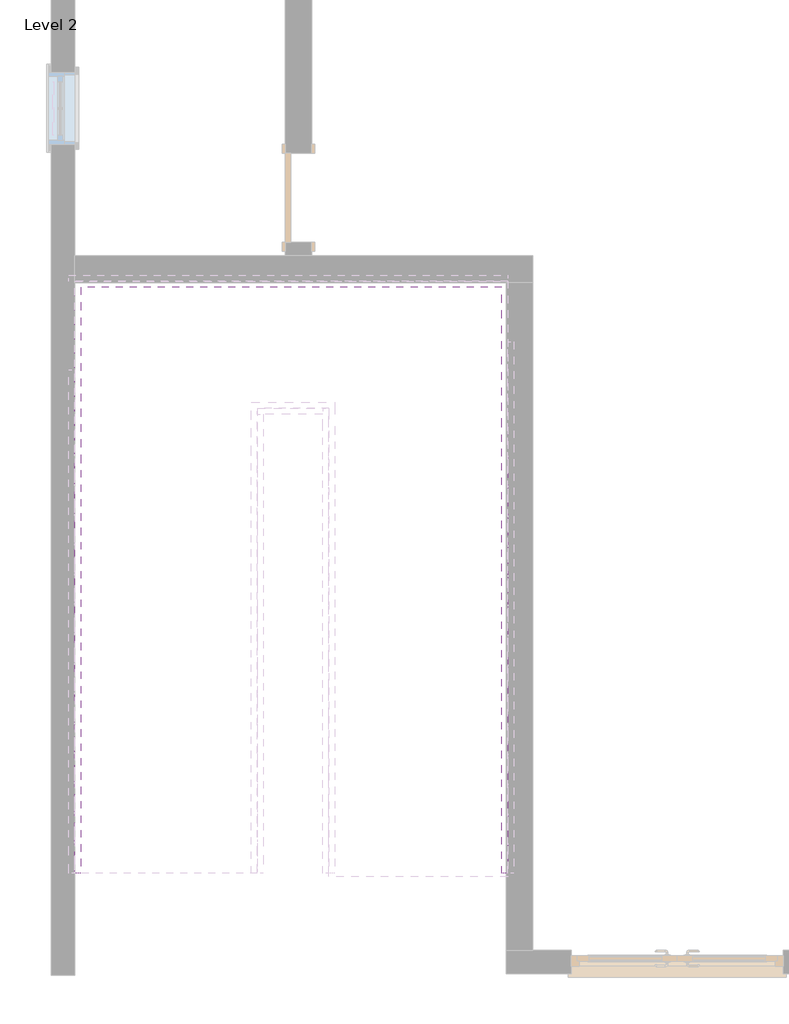
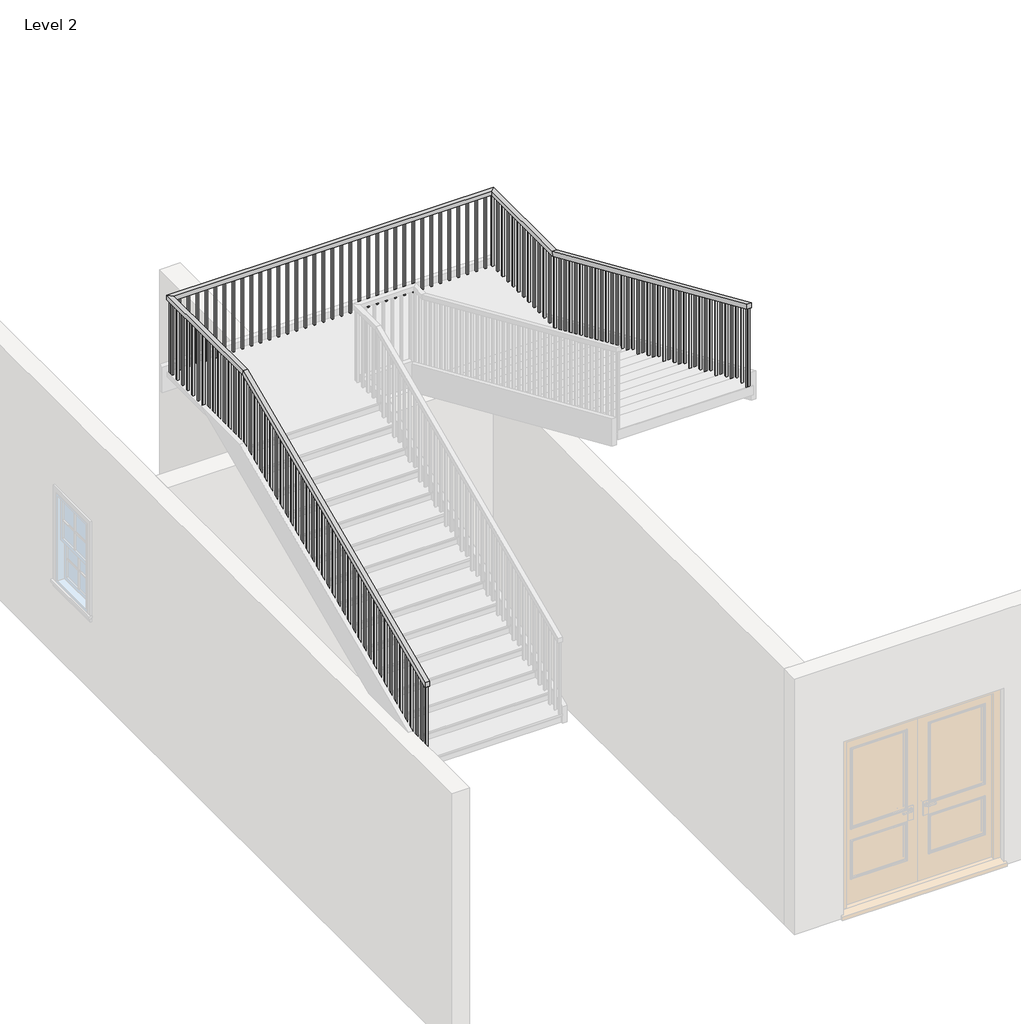
# One storey, part 3 of 4: 1 railing.
"""IFC4 building model written with IfcOpenShell, lengths in millimetres."""

from ifc_helpers import new_model, si_unit, frame, origin, place, context, project, spatial, polyline, outline, extrude, faceted_brep, element, save

model = new_model("IFC4")

# Units and contexts
model_context = context("Model", 3, world=origin())
ifc_project = project(units=[si_unit("LENGTHUNIT", "METRE", prefix="MILLI")], contexts=[model_context])

# Site, building, storey
site = spatial("IfcSite", under=ifc_project)
building = spatial("IfcBuilding", under=site)
storey = spatial("IfcBuildingStorey", under=building, Name="Level 2", Elevation=3048.0)

# Railing
placement = place(None, origin())
element("IfcRailing", 1, ObjectType="Handrail - Rectangular", at=placement, inside=storey, context=model_context, shape_type="SolidModel", body=[
    faceted_brep([(-7554.4415084, -6973.0610642, 6817.36), (-7554.4415084, -6973.0610642, 6761.8599828), (-7503.6415084, -6973.0610642, 6761.8599828), (-7503.6415084, -6973.0610642, 6817.36), (-7554.4415084, -3417.0610642, 8382.0), (-7554.4415084, -3406.3792071, 8331.2), (-7503.6415084, -3406.3792071, 8331.2), (-7503.6415084, -3417.0610642, 8382.0), (-7554.4415084, -1928.4217109, 8382.0), (-7554.4415084, -1928.4217109, 8331.2), (-7503.6415084, -1979.2217109, 8331.2), (-7503.6415084, -1979.2217109, 8382.0), (-3866.3290366, -1928.4217109, 8382.0), (-3866.3290366, -1928.4217109, 8331.2), (-3917.1290366, -1979.2217109, 8331.2), (-3917.1290366, -1979.2217109, 8382.0), (-3866.3290366, -3163.0610642, 8382.0), (-3866.3290366, -3173.7429214, 8331.2), (-3917.1290366, -3173.7429214, 8331.2), (-3917.1290366, -3163.0610642, 8382.0), (-3866.3290366, -6973.0610642, 10058.4), (-3917.1290366, -6973.0610642, 10058.4), (-3917.1290366, -6973.0610642, 10002.8999828), (-3866.3290366, -6973.0610642, 10002.8999828)], [[[0, 1, 2, 3]], [[1, 0, 4, 5]], [[2, 1, 5, 6]], [[3, 2, 6, 7]], [[0, 3, 7, 4]], [[5, 4, 8, 9]], [[6, 5, 9, 10]], [[7, 6, 10, 11]], [[4, 7, 11, 8]], [[9, 8, 12, 13]], [[10, 9, 13, 14]], [[11, 10, 14, 15]], [[8, 11, 15, 12]], [[13, 12, 16, 17]], [[14, 13, 17, 18]], [[15, 14, 18, 19]], [[12, 15, 19, 16]], [[20, 21, 22, 23]], [[17, 16, 20, 23]], [[18, 17, 23, 22]], [[19, 18, 22, 21]], [[16, 19, 21, 20]]]),
    extrude(outline(polyline([(-6922.6967109, 9980.7396674), (-6922.6967109, 9032.24), (-6941.7467109, 9032.24), (-6941.7467109, 9989.1216674), (-6922.6967109, 9980.7396674)])), frame((-3901.2540366, 0.0, 0.0), z_axis=(1.0, 0.0, 0.0), x_axis=(0.0, 1.0, 0.0)), (0.0, 0.0, 1.0), 19.05),
    extrude(outline(polyline([(-6821.0967109, 9936.0356674), (-6821.0967109, 9032.24), (-6840.1467109, 9032.24), (-6840.1467109, 9944.4176674), (-6821.0967109, 9936.0356674)])), frame((-3901.2540366, 0.0, 0.0), z_axis=(1.0, 0.0, 0.0), x_axis=(0.0, 1.0, 0.0)), (0.0, 0.0, 1.0), 19.05),
    extrude(outline(polyline([(-6719.4967109, 9891.3316674), (-6719.4967109, 9032.24), (-6738.5467109, 9032.24), (-6738.5467109, 9899.7136674), (-6719.4967109, 9891.3316674)])), frame((-3901.2540366, 0.0, 0.0), z_axis=(1.0, 0.0, 0.0), x_axis=(0.0, 1.0, 0.0)), (0.0, 0.0, 1.0), 19.05),
    extrude(outline(polyline([(-6617.8967109, 9846.6276674), (-6617.8967109, 8920.48), (-6636.9467109, 8920.48), (-6636.9467109, 9855.0096674), (-6617.8967109, 9846.6276674)])), frame((-3901.2540366, 0.0, 0.0), z_axis=(1.0, 0.0, 0.0), x_axis=(0.0, 1.0, 0.0)), (0.0, 0.0, 1.0), 19.05),
    extrude(outline(polyline([(-6516.2967109, 9801.9236674), (-6516.2967109, 8920.48), (-6535.3467109, 8920.48), (-6535.3467109, 9810.3056674), (-6516.2967109, 9801.9236674)])), frame((-3901.2540366, 0.0, 0.0), z_axis=(1.0, 0.0, 0.0), x_axis=(0.0, 1.0, 0.0)), (0.0, 0.0, 1.0), 19.05),
    extrude(outline(polyline([(-6414.6967109, 9757.2196674), (-6414.6967109, 8808.72), (-6433.7467109, 8808.72), (-6433.7467109, 9765.6016674), (-6414.6967109, 9757.2196674)])), frame((-3901.2540366, 0.0, 0.0), z_axis=(1.0, 0.0, 0.0), x_axis=(0.0, 1.0, 0.0)), (0.0, 0.0, 1.0), 19.05),
    extrude(outline(polyline([(-6313.0967109, 9712.5156674), (-6313.0967109, 8808.72), (-6332.1467109, 8808.72), (-6332.1467109, 9720.8976674), (-6313.0967109, 9712.5156674)])), frame((-3901.2540366, 0.0, 0.0), z_axis=(1.0, 0.0, 0.0), x_axis=(0.0, 1.0, 0.0)), (0.0, 0.0, 1.0), 19.05),
    extrude(outline(polyline([(-6211.4967109, 9667.8116674), (-6211.4967109, 8808.72), (-6230.5467109, 8808.72), (-6230.5467109, 9676.1936674), (-6211.4967109, 9667.8116674)])), frame((-3901.2540366, 0.0, 0.0), z_axis=(1.0, 0.0, 0.0), x_axis=(0.0, 1.0, 0.0)), (0.0, 0.0, 1.0), 19.05),
    extrude(outline(polyline([(-6109.8967109, 9623.1076674), (-6109.8967109, 8696.96), (-6128.9467109, 8696.96), (-6128.9467109, 9631.4896674), (-6109.8967109, 9623.1076674)])), frame((-3901.2540366, 0.0, 0.0), z_axis=(1.0, 0.0, 0.0), x_axis=(0.0, 1.0, 0.0)), (0.0, 0.0, 1.0), 19.05),
    extrude(outline(polyline([(-6008.2967109, 9578.4036674), (-6008.2967109, 8696.96), (-6027.3467109, 8696.96), (-6027.3467109, 9586.7856674), (-6008.2967109, 9578.4036674)])), frame((-3901.2540366, 0.0, 0.0), z_axis=(1.0, 0.0, 0.0), x_axis=(0.0, 1.0, 0.0)), (0.0, 0.0, 1.0), 19.05),
    extrude(outline(polyline([(-5906.6967109, 9533.6996674), (-5906.6967109, 8585.2), (-5925.7467109, 8585.2), (-5925.7467109, 9542.0816674), (-5906.6967109, 9533.6996674)])), frame((-3901.2540366, 0.0, 0.0), z_axis=(1.0, 0.0, 0.0), x_axis=(0.0, 1.0, 0.0)), (0.0, 0.0, 1.0), 19.05),
    extrude(outline(polyline([(-5805.0967109, 9488.9956674), (-5805.0967109, 8585.2), (-5824.1467109, 8585.2), (-5824.1467109, 9497.3776674), (-5805.0967109, 9488.9956674)])), frame((-3901.2540366, 0.0, 0.0), z_axis=(1.0, 0.0, 0.0), x_axis=(0.0, 1.0, 0.0)), (0.0, 0.0, 1.0), 19.05),
    extrude(outline(polyline([(-5703.4967109, 9444.2916674), (-5703.4967109, 8585.2), (-5722.5467109, 8585.2), (-5722.5467109, 9452.6736674), (-5703.4967109, 9444.2916674)])), frame((-3901.2540366, 0.0, 0.0), z_axis=(1.0, 0.0, 0.0), x_axis=(0.0, 1.0, 0.0)), (0.0, 0.0, 1.0), 19.05),
    extrude(outline(polyline([(-5601.8967109, 9399.5876674), (-5601.8967109, 8473.44), (-5620.9467109, 8473.44), (-5620.9467109, 9407.9696674), (-5601.8967109, 9399.5876674)])), frame((-3901.2540366, 0.0, 0.0), z_axis=(1.0, 0.0, 0.0), x_axis=(0.0, 1.0, 0.0)), (0.0, 0.0, 1.0), 19.05),
    extrude(outline(polyline([(-5500.2967109, 9354.8836674), (-5500.2967109, 8473.44), (-5519.3467109, 8473.44), (-5519.3467109, 9363.2656674), (-5500.2967109, 9354.8836674)])), frame((-3901.2540366, 0.0, 0.0), z_axis=(1.0, 0.0, 0.0), x_axis=(0.0, 1.0, 0.0)), (0.0, 0.0, 1.0), 19.05),
    extrude(outline(polyline([(-5398.6967109, 9310.1796674), (-5398.6967109, 8361.68), (-5417.7467109, 8361.68), (-5417.7467109, 9318.5616674), (-5398.6967109, 9310.1796674)])), frame((-3901.2540366, 0.0, 0.0), z_axis=(1.0, 0.0, 0.0), x_axis=(0.0, 1.0, 0.0)), (0.0, 0.0, 1.0), 19.05),
    extrude(outline(polyline([(-5297.0967109, 9265.4756674), (-5297.0967109, 8361.68), (-5316.1467109, 8361.68), (-5316.1467109, 9273.8576674), (-5297.0967109, 9265.4756674)])), frame((-3901.2540366, 0.0, 0.0), z_axis=(1.0, 0.0, 0.0), x_axis=(0.0, 1.0, 0.0)), (0.0, 0.0, 1.0), 19.05),
    extrude(outline(polyline([(-5195.4967109, 9220.7716674), (-5195.4967109, 8361.68), (-5214.5467109, 8361.68), (-5214.5467109, 9229.1536674), (-5195.4967109, 9220.7716674)])), frame((-3901.2540366, 0.0, 0.0), z_axis=(1.0, 0.0, 0.0), x_axis=(0.0, 1.0, 0.0)), (0.0, 0.0, 1.0), 19.05),
    extrude(outline(polyline([(-5093.8967109, 9176.0676674), (-5093.8967109, 8249.92), (-5112.9467109, 8249.92), (-5112.9467109, 9184.4496674), (-5093.8967109, 9176.0676674)])), frame((-3901.2540366, 0.0, 0.0), z_axis=(1.0, 0.0, 0.0), x_axis=(0.0, 1.0, 0.0)), (0.0, 0.0, 1.0), 19.05),
    extrude(outline(polyline([(-4992.2967109, 9131.3636674), (-4992.2967109, 8249.92), (-5011.3467109, 8249.92), (-5011.3467109, 9139.7456674), (-4992.2967109, 9131.3636674)])), frame((-3901.2540366, 0.0, 0.0), z_axis=(1.0, 0.0, 0.0), x_axis=(0.0, 1.0, 0.0)), (0.0, 0.0, 1.0), 19.05),
    extrude(outline(polyline([(-4890.6967109, 9086.6596674), (-4890.6967109, 8138.16), (-4909.7467109, 8138.16), (-4909.7467109, 9095.0416674), (-4890.6967109, 9086.6596674)])), frame((-3901.2540366, 0.0, 0.0), z_axis=(1.0, 0.0, 0.0), x_axis=(0.0, 1.0, 0.0)), (0.0, 0.0, 1.0), 19.05),
    extrude(outline(polyline([(-4789.0967109, 9041.9556674), (-4789.0967109, 8138.16), (-4808.1467109, 8138.16), (-4808.1467109, 9050.3376674), (-4789.0967109, 9041.9556674)])), frame((-3901.2540366, 0.0, 0.0), z_axis=(1.0, 0.0, 0.0), x_axis=(0.0, 1.0, 0.0)), (0.0, 0.0, 1.0), 19.05),
    extrude(outline(polyline([(-4687.4967109, 8997.2516674), (-4687.4967109, 8138.16), (-4706.5467109, 8138.16), (-4706.5467109, 9005.6336674), (-4687.4967109, 8997.2516674)])), frame((-3901.2540366, 0.0, 0.0), z_axis=(1.0, 0.0, 0.0), x_axis=(0.0, 1.0, 0.0)), (0.0, 0.0, 1.0), 19.05),
    extrude(outline(polyline([(-4585.8967109, 8952.5476674), (-4585.8967109, 8026.4), (-4604.9467109, 8026.4), (-4604.9467109, 8960.9296674), (-4585.8967109, 8952.5476674)])), frame((-3901.2540366, 0.0, 0.0), z_axis=(1.0, 0.0, 0.0), x_axis=(0.0, 1.0, 0.0)), (0.0, 0.0, 1.0), 19.05),
    extrude(outline(polyline([(-4484.2967109, 8907.8436674), (-4484.2967109, 8026.4), (-4503.3467109, 8026.4), (-4503.3467109, 8916.2256674), (-4484.2967109, 8907.8436674)])), frame((-3901.2540366, 0.0, 0.0), z_axis=(1.0, 0.0, 0.0), x_axis=(0.0, 1.0, 0.0)), (0.0, 0.0, 1.0), 19.05),
    extrude(outline(polyline([(-4382.6967109, 8863.1396674), (-4382.6967109, 7914.64), (-4401.7467109, 7914.64), (-4401.7467109, 8871.5216674), (-4382.6967109, 8863.1396674)])), frame((-3901.2540366, 0.0, 0.0), z_axis=(1.0, 0.0, 0.0), x_axis=(0.0, 1.0, 0.0)), (0.0, 0.0, 1.0), 19.05),
    extrude(outline(polyline([(-4281.0967109, 8818.4356674), (-4281.0967109, 7914.64), (-4300.1467109, 7914.64), (-4300.1467109, 8826.8176674), (-4281.0967109, 8818.4356674)])), frame((-3901.2540366, 0.0, 0.0), z_axis=(1.0, 0.0, 0.0), x_axis=(0.0, 1.0, 0.0)), (0.0, 0.0, 1.0), 19.05),
    extrude(outline(polyline([(-4179.4967109, 8773.7316674), (-4179.4967109, 7914.64), (-4198.5467109, 7914.64), (-4198.5467109, 8782.1136674), (-4179.4967109, 8773.7316674)])), frame((-3901.2540366, 0.0, 0.0), z_axis=(1.0, 0.0, 0.0), x_axis=(0.0, 1.0, 0.0)), (0.0, 0.0, 1.0), 19.05),
    extrude(outline(polyline([(-4077.8967109, 8729.0276674), (-4077.8967109, 7802.88), (-4096.9467109, 7802.88), (-4096.9467109, 8737.4096674), (-4077.8967109, 8729.0276674)])), frame((-3901.2540366, 0.0, 0.0), z_axis=(1.0, 0.0, 0.0), x_axis=(0.0, 1.0, 0.0)), (0.0, 0.0, 1.0), 19.05),
    extrude(outline(polyline([(-3976.2967109, 8684.3236674), (-3976.2967109, 7802.88), (-3995.3467109, 7802.88), (-3995.3467109, 8692.7056674), (-3976.2967109, 8684.3236674)])), frame((-3901.2540366, 0.0, 0.0), z_axis=(1.0, 0.0, 0.0), x_axis=(0.0, 1.0, 0.0)), (0.0, 0.0, 1.0), 19.05),
    extrude(outline(polyline([(-3874.6967109, 8639.6196674), (-3874.6967109, 7691.12), (-3893.7467109, 7691.12), (-3893.7467109, 8648.0016674), (-3874.6967109, 8639.6196674)])), frame((-3901.2540366, 0.0, 0.0), z_axis=(1.0, 0.0, 0.0), x_axis=(0.0, 1.0, 0.0)), (0.0, 0.0, 1.0), 19.05),
    extrude(outline(polyline([(-3773.0967109, 8594.9156674), (-3773.0967109, 7691.12), (-3792.1467109, 7691.12), (-3792.1467109, 8603.2976674), (-3773.0967109, 8594.9156674)])), frame((-3901.2540366, 0.0, 0.0), z_axis=(1.0, 0.0, 0.0), x_axis=(0.0, 1.0, 0.0)), (0.0, 0.0, 1.0), 19.05),
    extrude(outline(polyline([(-3671.4967109, 8550.2116674), (-3671.4967109, 7691.12), (-3690.5467109, 7691.12), (-3690.5467109, 8558.5936674), (-3671.4967109, 8550.2116674)])), frame((-3901.2540366, 0.0, 0.0), z_axis=(1.0, 0.0, 0.0), x_axis=(0.0, 1.0, 0.0)), (0.0, 0.0, 1.0), 19.05),
    extrude(outline(polyline([(-3569.8967109, 8505.5076674), (-3569.8967109, 7579.36), (-3588.9467109, 7579.36), (-3588.9467109, 8513.8896674), (-3569.8967109, 8505.5076674)])), frame((-3901.2540366, 0.0, 0.0), z_axis=(1.0, 0.0, 0.0), x_axis=(0.0, 1.0, 0.0)), (0.0, 0.0, 1.0), 19.05),
    extrude(outline(polyline([(-3468.2967109, 8460.8036674), (-3468.2967109, 7579.36), (-3487.3467109, 7579.36), (-3487.3467109, 8469.1856674), (-3468.2967109, 8460.8036674)])), frame((-3901.2540366, 0.0, 0.0), z_axis=(1.0, 0.0, 0.0), x_axis=(0.0, 1.0, 0.0)), (0.0, 0.0, 1.0), 19.05),
    extrude(outline(polyline([(-3366.6967109, 8416.0996674), (-3366.6967109, 7467.6), (-3385.7467109, 7467.6), (-3385.7467109, 8424.4816674), (-3366.6967109, 8416.0996674)])), frame((-3901.2540366, 0.0, 0.0), z_axis=(1.0, 0.0, 0.0), x_axis=(0.0, 1.0, 0.0)), (0.0, 0.0, 1.0), 19.05),
    extrude(outline(polyline([(-3265.0967109, 8371.3956674), (-3265.0967109, 7467.6), (-3284.1467109, 7467.6), (-3284.1467109, 8379.7776674), (-3265.0967109, 8371.3956674)])), frame((-3901.2540366, 0.0, 0.0), z_axis=(1.0, 0.0, 0.0), x_axis=(0.0, 1.0, 0.0)), (0.0, 0.0, 1.0), 19.05),
    extrude(outline(polyline([(-3163.4967109, 8326.6916674), (-3163.4967109, 7467.6), (-3182.5467109, 7467.6), (-3182.5467109, 8335.0736674), (-3163.4967109, 8326.6916674)])), frame((-3901.2540366, 0.0, 0.0), z_axis=(1.0, 0.0, 0.0), x_axis=(0.0, 1.0, 0.0)), (0.0, 0.0, 1.0), 19.05),
    extrude(outline(polyline([(-3882.2040366, -3061.8967109), (-3882.2040366, -3080.9467109), (-3901.2540366, -3080.9467109), (-3901.2540366, -3061.8967109), (-3882.2040366, -3061.8967109)])), frame((0.0, 0.0, 7467.6), z_axis=(0.0, 0.0, 1.0), x_axis=(1.0, 0.0, 0.0)), (0.0, 0.0, 1.0), 863.6),
    extrude(outline(polyline([(-3882.2040366, -2960.2967109), (-3882.2040366, -2979.3467109), (-3901.2540366, -2979.3467109), (-3901.2540366, -2960.2967109), (-3882.2040366, -2960.2967109)])), frame((0.0, 0.0, 7467.6), z_axis=(0.0, 0.0, 1.0), x_axis=(1.0, 0.0, 0.0)), (0.0, 0.0, 1.0), 863.6),
    extrude(outline(polyline([(-3882.2040366, -2858.6967109), (-3882.2040366, -2877.7467109), (-3901.2540366, -2877.7467109), (-3901.2540366, -2858.6967109), (-3882.2040366, -2858.6967109)])), frame((0.0, 0.0, 7467.6), z_axis=(0.0, 0.0, 1.0), x_axis=(1.0, 0.0, 0.0)), (0.0, 0.0, 1.0), 863.6),
    extrude(outline(polyline([(-3882.2040366, -2757.0967109), (-3882.2040366, -2776.1467109), (-3901.2540366, -2776.1467109), (-3901.2540366, -2757.0967109), (-3882.2040366, -2757.0967109)])), frame((0.0, 0.0, 7467.6), z_axis=(0.0, 0.0, 1.0), x_axis=(1.0, 0.0, 0.0)), (0.0, 0.0, 1.0), 863.6),
    extrude(outline(polyline([(-3882.2040366, -2655.4967109), (-3882.2040366, -2674.5467109), (-3901.2540366, -2674.5467109), (-3901.2540366, -2655.4967109), (-3882.2040366, -2655.4967109)])), frame((0.0, 0.0, 7467.6), z_axis=(0.0, 0.0, 1.0), x_axis=(1.0, 0.0, 0.0)), (0.0, 0.0, 1.0), 863.6),
    extrude(outline(polyline([(-3882.2040366, -2553.8967109), (-3882.2040366, -2572.9467109), (-3901.2540366, -2572.9467109), (-3901.2540366, -2553.8967109), (-3882.2040366, -2553.8967109)])), frame((0.0, 0.0, 7467.6), z_axis=(0.0, 0.0, 1.0), x_axis=(1.0, 0.0, 0.0)), (0.0, 0.0, 1.0), 863.6),
    extrude(outline(polyline([(-3882.2040366, -2452.2967109), (-3882.2040366, -2471.3467109), (-3901.2540366, -2471.3467109), (-3901.2540366, -2452.2967109), (-3882.2040366, -2452.2967109)])), frame((0.0, 0.0, 7467.6), z_axis=(0.0, 0.0, 1.0), x_axis=(1.0, 0.0, 0.0)), (0.0, 0.0, 1.0), 863.6),
    extrude(outline(polyline([(-3882.2040366, -2350.6967109), (-3882.2040366, -2369.7467109), (-3901.2540366, -2369.7467109), (-3901.2540366, -2350.6967109), (-3882.2040366, -2350.6967109)])), frame((0.0, 0.0, 7467.6), z_axis=(0.0, 0.0, 1.0), x_axis=(1.0, 0.0, 0.0)), (0.0, 0.0, 1.0), 863.6),
    extrude(outline(polyline([(-3882.2040366, -2249.0967109), (-3882.2040366, -2268.1467109), (-3901.2540366, -2268.1467109), (-3901.2540366, -2249.0967109), (-3882.2040366, -2249.0967109)])), frame((0.0, 0.0, 7467.6), z_axis=(0.0, 0.0, 1.0), x_axis=(1.0, 0.0, 0.0)), (0.0, 0.0, 1.0), 863.6),
    extrude(outline(polyline([(-3882.2040366, -2147.4967109), (-3882.2040366, -2166.5467109), (-3901.2540366, -2166.5467109), (-3901.2540366, -2147.4967109), (-3882.2040366, -2147.4967109)])), frame((0.0, 0.0, 7467.6), z_axis=(0.0, 0.0, 1.0), x_axis=(1.0, 0.0, 0.0)), (0.0, 0.0, 1.0), 863.6),
    extrude(outline(polyline([(-3882.2040366, -2045.8967109), (-3882.2040366, -2064.9467109), (-3901.2540366, -2064.9467109), (-3901.2540366, -2045.8967109), (-3882.2040366, -2045.8967109)])), frame((0.0, 0.0, 7467.6), z_axis=(0.0, 0.0, 1.0), x_axis=(1.0, 0.0, 0.0)), (0.0, 0.0, 1.0), 863.6),
    extrude(outline(polyline([(-3982.5665084, -1944.2967109), (-3963.5165084, -1944.2967109), (-3963.5165084, -1963.3467109), (-3982.5665084, -1963.3467109), (-3982.5665084, -1944.2967109)])), frame((0.0, 0.0, 7467.6), z_axis=(0.0, 0.0, 1.0), x_axis=(1.0, 0.0, 0.0)), (0.0, 0.0, 1.0), 863.6),
    extrude(outline(polyline([(-4084.1665084, -1944.2967109), (-4065.1165084, -1944.2967109), (-4065.1165084, -1963.3467109), (-4084.1665084, -1963.3467109), (-4084.1665084, -1944.2967109)])), frame((0.0, 0.0, 7467.6), z_axis=(0.0, 0.0, 1.0), x_axis=(1.0, 0.0, 0.0)), (0.0, 0.0, 1.0), 863.6),
    extrude(outline(polyline([(-4185.7665084, -1944.2967109), (-4166.7165084, -1944.2967109), (-4166.7165084, -1963.3467109), (-4185.7665084, -1963.3467109), (-4185.7665084, -1944.2967109)])), frame((0.0, 0.0, 7467.6), z_axis=(0.0, 0.0, 1.0), x_axis=(1.0, 0.0, 0.0)), (0.0, 0.0, 1.0), 863.6),
    extrude(outline(polyline([(-4287.3665084, -1944.2967109), (-4268.3165084, -1944.2967109), (-4268.3165084, -1963.3467109), (-4287.3665084, -1963.3467109), (-4287.3665084, -1944.2967109)])), frame((0.0, 0.0, 7467.6), z_axis=(0.0, 0.0, 1.0), x_axis=(1.0, 0.0, 0.0)), (0.0, 0.0, 1.0), 863.6),
    extrude(outline(polyline([(-4388.9665084, -1944.2967109), (-4369.9165084, -1944.2967109), (-4369.9165084, -1963.3467109), (-4388.9665084, -1963.3467109), (-4388.9665084, -1944.2967109)])), frame((0.0, 0.0, 7467.6), z_axis=(0.0, 0.0, 1.0), x_axis=(1.0, 0.0, 0.0)), (0.0, 0.0, 1.0), 863.6),
    extrude(outline(polyline([(-4490.5665084, -1944.2967109), (-4471.5165084, -1944.2967109), (-4471.5165084, -1963.3467109), (-4490.5665084, -1963.3467109), (-4490.5665084, -1944.2967109)])), frame((0.0, 0.0, 7467.6), z_axis=(0.0, 0.0, 1.0), x_axis=(1.0, 0.0, 0.0)), (0.0, 0.0, 1.0), 863.6),
    extrude(outline(polyline([(-4592.1665084, -1944.2967109), (-4573.1165084, -1944.2967109), (-4573.1165084, -1963.3467109), (-4592.1665084, -1963.3467109), (-4592.1665084, -1944.2967109)])), frame((0.0, 0.0, 7467.6), z_axis=(0.0, 0.0, 1.0), x_axis=(1.0, 0.0, 0.0)), (0.0, 0.0, 1.0), 863.6),
    extrude(outline(polyline([(-4693.7665084, -1944.2967109), (-4674.7165084, -1944.2967109), (-4674.7165084, -1963.3467109), (-4693.7665084, -1963.3467109), (-4693.7665084, -1944.2967109)])), frame((0.0, 0.0, 7467.6), z_axis=(0.0, 0.0, 1.0), x_axis=(1.0, 0.0, 0.0)), (0.0, 0.0, 1.0), 863.6),
    extrude(outline(polyline([(-4795.3665084, -1944.2967109), (-4776.3165084, -1944.2967109), (-4776.3165084, -1963.3467109), (-4795.3665084, -1963.3467109), (-4795.3665084, -1944.2967109)])), frame((0.0, 0.0, 7467.6), z_axis=(0.0, 0.0, 1.0), x_axis=(1.0, 0.0, 0.0)), (0.0, 0.0, 1.0), 863.6),
    extrude(outline(polyline([(-4896.9665084, -1944.2967109), (-4877.9165084, -1944.2967109), (-4877.9165084, -1963.3467109), (-4896.9665084, -1963.3467109), (-4896.9665084, -1944.2967109)])), frame((0.0, 0.0, 7467.6), z_axis=(0.0, 0.0, 1.0), x_axis=(1.0, 0.0, 0.0)), (0.0, 0.0, 1.0), 863.6),
    extrude(outline(polyline([(-4998.5665084, -1944.2967109), (-4979.5165084, -1944.2967109), (-4979.5165084, -1963.3467109), (-4998.5665084, -1963.3467109), (-4998.5665084, -1944.2967109)])), frame((0.0, 0.0, 7467.6), z_axis=(0.0, 0.0, 1.0), x_axis=(1.0, 0.0, 0.0)), (0.0, 0.0, 1.0), 863.6),
    extrude(outline(polyline([(-5100.1665084, -1944.2967109), (-5081.1165084, -1944.2967109), (-5081.1165084, -1963.3467109), (-5100.1665084, -1963.3467109), (-5100.1665084, -1944.2967109)])), frame((0.0, 0.0, 7467.6), z_axis=(0.0, 0.0, 1.0), x_axis=(1.0, 0.0, 0.0)), (0.0, 0.0, 1.0), 863.6),
    extrude(outline(polyline([(-5201.7665084, -1944.2967109), (-5182.7165084, -1944.2967109), (-5182.7165084, -1963.3467109), (-5201.7665084, -1963.3467109), (-5201.7665084, -1944.2967109)])), frame((0.0, 0.0, 7467.6), z_axis=(0.0, 0.0, 1.0), x_axis=(1.0, 0.0, 0.0)), (0.0, 0.0, 1.0), 863.6),
    extrude(outline(polyline([(-5303.3665084, -1944.2967109), (-5284.3165084, -1944.2967109), (-5284.3165084, -1963.3467109), (-5303.3665084, -1963.3467109), (-5303.3665084, -1944.2967109)])), frame((0.0, 0.0, 7467.6), z_axis=(0.0, 0.0, 1.0), x_axis=(1.0, 0.0, 0.0)), (0.0, 0.0, 1.0), 863.6),
    extrude(outline(polyline([(-5404.9665084, -1944.2967109), (-5385.9165084, -1944.2967109), (-5385.9165084, -1963.3467109), (-5404.9665084, -1963.3467109), (-5404.9665084, -1944.2967109)])), frame((0.0, 0.0, 7467.6), z_axis=(0.0, 0.0, 1.0), x_axis=(1.0, 0.0, 0.0)), (0.0, 0.0, 1.0), 863.6),
    extrude(outline(polyline([(-5506.5665084, -1944.2967109), (-5487.5165084, -1944.2967109), (-5487.5165084, -1963.3467109), (-5506.5665084, -1963.3467109), (-5506.5665084, -1944.2967109)])), frame((0.0, 0.0, 7467.6), z_axis=(0.0, 0.0, 1.0), x_axis=(1.0, 0.0, 0.0)), (0.0, 0.0, 1.0), 863.6),
    extrude(outline(polyline([(-5608.1665084, -1944.2967109), (-5589.1165084, -1944.2967109), (-5589.1165084, -1963.3467109), (-5608.1665084, -1963.3467109), (-5608.1665084, -1944.2967109)])), frame((0.0, 0.0, 7467.6), z_axis=(0.0, 0.0, 1.0), x_axis=(1.0, 0.0, 0.0)), (0.0, 0.0, 1.0), 863.6),
    extrude(outline(polyline([(-5709.7665084, -1944.2967109), (-5690.7165084, -1944.2967109), (-5690.7165084, -1963.3467109), (-5709.7665084, -1963.3467109), (-5709.7665084, -1944.2967109)])), frame((0.0, 0.0, 7467.6), z_axis=(0.0, 0.0, 1.0), x_axis=(1.0, 0.0, 0.0)), (0.0, 0.0, 1.0), 863.6),
    extrude(outline(polyline([(-5811.3665084, -1944.2967109), (-5792.3165084, -1944.2967109), (-5792.3165084, -1963.3467109), (-5811.3665084, -1963.3467109), (-5811.3665084, -1944.2967109)])), frame((0.0, 0.0, 7467.6), z_axis=(0.0, 0.0, 1.0), x_axis=(1.0, 0.0, 0.0)), (0.0, 0.0, 1.0), 863.6),
    extrude(outline(polyline([(-5912.9665084, -1944.2967109), (-5893.9165084, -1944.2967109), (-5893.9165084, -1963.3467109), (-5912.9665084, -1963.3467109), (-5912.9665084, -1944.2967109)])), frame((0.0, 0.0, 7467.6), z_axis=(0.0, 0.0, 1.0), x_axis=(1.0, 0.0, 0.0)), (0.0, 0.0, 1.0), 863.6),
    extrude(outline(polyline([(-6014.5665084, -1944.2967109), (-5995.5165084, -1944.2967109), (-5995.5165084, -1963.3467109), (-6014.5665084, -1963.3467109), (-6014.5665084, -1944.2967109)])), frame((0.0, 0.0, 7467.6), z_axis=(0.0, 0.0, 1.0), x_axis=(1.0, 0.0, 0.0)), (0.0, 0.0, 1.0), 863.6),
    extrude(outline(polyline([(-6116.1665084, -1944.2967109), (-6097.1165084, -1944.2967109), (-6097.1165084, -1963.3467109), (-6116.1665084, -1963.3467109), (-6116.1665084, -1944.2967109)])), frame((0.0, 0.0, 7467.6), z_axis=(0.0, 0.0, 1.0), x_axis=(1.0, 0.0, 0.0)), (0.0, 0.0, 1.0), 863.6),
    extrude(outline(polyline([(-6217.7665084, -1944.2967109), (-6198.7165084, -1944.2967109), (-6198.7165084, -1963.3467109), (-6217.7665084, -1963.3467109), (-6217.7665084, -1944.2967109)])), frame((0.0, 0.0, 7467.6), z_axis=(0.0, 0.0, 1.0), x_axis=(1.0, 0.0, 0.0)), (0.0, 0.0, 1.0), 863.6),
    extrude(outline(polyline([(-6319.3665084, -1944.2967109), (-6300.3165084, -1944.2967109), (-6300.3165084, -1963.3467109), (-6319.3665084, -1963.3467109), (-6319.3665084, -1944.2967109)])), frame((0.0, 0.0, 7467.6), z_axis=(0.0, 0.0, 1.0), x_axis=(1.0, 0.0, 0.0)), (0.0, 0.0, 1.0), 863.6),
    extrude(outline(polyline([(-6420.9665084, -1944.2967109), (-6401.9165084, -1944.2967109), (-6401.9165084, -1963.3467109), (-6420.9665084, -1963.3467109), (-6420.9665084, -1944.2967109)])), frame((0.0, 0.0, 7467.6), z_axis=(0.0, 0.0, 1.0), x_axis=(1.0, 0.0, 0.0)), (0.0, 0.0, 1.0), 863.6),
    extrude(outline(polyline([(-6522.5665084, -1944.2967109), (-6503.5165084, -1944.2967109), (-6503.5165084, -1963.3467109), (-6522.5665084, -1963.3467109), (-6522.5665084, -1944.2967109)])), frame((0.0, 0.0, 7467.6), z_axis=(0.0, 0.0, 1.0), x_axis=(1.0, 0.0, 0.0)), (0.0, 0.0, 1.0), 863.6),
    extrude(outline(polyline([(-6624.1665084, -1944.2967109), (-6605.1165084, -1944.2967109), (-6605.1165084, -1963.3467109), (-6624.1665084, -1963.3467109), (-6624.1665084, -1944.2967109)])), frame((0.0, 0.0, 7467.6), z_axis=(0.0, 0.0, 1.0), x_axis=(1.0, 0.0, 0.0)), (0.0, 0.0, 1.0), 863.6),
    extrude(outline(polyline([(-6725.7665084, -1944.2967109), (-6706.7165084, -1944.2967109), (-6706.7165084, -1963.3467109), (-6725.7665084, -1963.3467109), (-6725.7665084, -1944.2967109)])), frame((0.0, 0.0, 7467.6), z_axis=(0.0, 0.0, 1.0), x_axis=(1.0, 0.0, 0.0)), (0.0, 0.0, 1.0), 863.6),
    extrude(outline(polyline([(-6827.3665084, -1944.2967109), (-6808.3165084, -1944.2967109), (-6808.3165084, -1963.3467109), (-6827.3665084, -1963.3467109), (-6827.3665084, -1944.2967109)])), frame((0.0, 0.0, 7467.6), z_axis=(0.0, 0.0, 1.0), x_axis=(1.0, 0.0, 0.0)), (0.0, 0.0, 1.0), 863.6),
    extrude(outline(polyline([(-6928.9665084, -1944.2967109), (-6909.9165084, -1944.2967109), (-6909.9165084, -1963.3467109), (-6928.9665084, -1963.3467109), (-6928.9665084, -1944.2967109)])), frame((0.0, 0.0, 7467.6), z_axis=(0.0, 0.0, 1.0), x_axis=(1.0, 0.0, 0.0)), (0.0, 0.0, 1.0), 863.6),
    extrude(outline(polyline([(-7030.5665084, -1944.2967109), (-7011.5165084, -1944.2967109), (-7011.5165084, -1963.3467109), (-7030.5665084, -1963.3467109), (-7030.5665084, -1944.2967109)])), frame((0.0, 0.0, 7467.6), z_axis=(0.0, 0.0, 1.0), x_axis=(1.0, 0.0, 0.0)), (0.0, 0.0, 1.0), 863.6),
    extrude(outline(polyline([(-7132.1665084, -1944.2967109), (-7113.1165084, -1944.2967109), (-7113.1165084, -1963.3467109), (-7132.1665084, -1963.3467109), (-7132.1665084, -1944.2967109)])), frame((0.0, 0.0, 7467.6), z_axis=(0.0, 0.0, 1.0), x_axis=(1.0, 0.0, 0.0)), (0.0, 0.0, 1.0), 863.6),
    extrude(outline(polyline([(-7233.7665084, -1944.2967109), (-7214.7165084, -1944.2967109), (-7214.7165084, -1963.3467109), (-7233.7665084, -1963.3467109), (-7233.7665084, -1944.2967109)])), frame((0.0, 0.0, 7467.6), z_axis=(0.0, 0.0, 1.0), x_axis=(1.0, 0.0, 0.0)), (0.0, 0.0, 1.0), 863.6),
    extrude(outline(polyline([(-7335.3665084, -1944.2967109), (-7316.3165084, -1944.2967109), (-7316.3165084, -1963.3467109), (-7335.3665084, -1963.3467109), (-7335.3665084, -1944.2967109)])), frame((0.0, 0.0, 7467.6), z_axis=(0.0, 0.0, 1.0), x_axis=(1.0, 0.0, 0.0)), (0.0, 0.0, 1.0), 863.6),
    extrude(outline(polyline([(-7436.9665084, -1944.2967109), (-7417.9165084, -1944.2967109), (-7417.9165084, -1963.3467109), (-7436.9665084, -1963.3467109), (-7436.9665084, -1944.2967109)])), frame((0.0, 0.0, 7467.6), z_axis=(0.0, 0.0, 1.0), x_axis=(1.0, 0.0, 0.0)), (0.0, 0.0, 1.0), 863.6),
    extrude(outline(polyline([(-7538.5665084, -2004.1860642), (-7538.5665084, -1985.1360642), (-7519.5165084, -1985.1360642), (-7519.5165084, -2004.1860642), (-7538.5665084, -2004.1860642)])), frame((0.0, 0.0, 7467.6), z_axis=(0.0, 0.0, 1.0), x_axis=(1.0, 0.0, 0.0)), (0.0, 0.0, 1.0), 863.6),
    extrude(outline(polyline([(-7538.5665084, -2105.7860642), (-7538.5665084, -2086.7360642), (-7519.5165084, -2086.7360642), (-7519.5165084, -2105.7860642), (-7538.5665084, -2105.7860642)])), frame((0.0, 0.0, 7467.6), z_axis=(0.0, 0.0, 1.0), x_axis=(1.0, 0.0, 0.0)), (0.0, 0.0, 1.0), 863.6),
    extrude(outline(polyline([(-7538.5665084, -2207.3860642), (-7538.5665084, -2188.3360642), (-7519.5165084, -2188.3360642), (-7519.5165084, -2207.3860642), (-7538.5665084, -2207.3860642)])), frame((0.0, 0.0, 7467.6), z_axis=(0.0, 0.0, 1.0), x_axis=(1.0, 0.0, 0.0)), (0.0, 0.0, 1.0), 863.6),
    extrude(outline(polyline([(-7538.5665084, -2308.9860642), (-7538.5665084, -2289.9360642), (-7519.5165084, -2289.9360642), (-7519.5165084, -2308.9860642), (-7538.5665084, -2308.9860642)])), frame((0.0, 0.0, 7467.6), z_axis=(0.0, 0.0, 1.0), x_axis=(1.0, 0.0, 0.0)), (0.0, 0.0, 1.0), 863.6),
    extrude(outline(polyline([(-7538.5665084, -2410.5860642), (-7538.5665084, -2391.5360642), (-7519.5165084, -2391.5360642), (-7519.5165084, -2410.5860642), (-7538.5665084, -2410.5860642)])), frame((0.0, 0.0, 7467.6), z_axis=(0.0, 0.0, 1.0), x_axis=(1.0, 0.0, 0.0)), (0.0, 0.0, 1.0), 863.6),
    extrude(outline(polyline([(-7538.5665084, -2512.1860642), (-7538.5665084, -2493.1360642), (-7519.5165084, -2493.1360642), (-7519.5165084, -2512.1860642), (-7538.5665084, -2512.1860642)])), frame((0.0, 0.0, 7467.6), z_axis=(0.0, 0.0, 1.0), x_axis=(1.0, 0.0, 0.0)), (0.0, 0.0, 1.0), 863.6),
    extrude(outline(polyline([(-7538.5665084, -2613.7860642), (-7538.5665084, -2594.7360642), (-7519.5165084, -2594.7360642), (-7519.5165084, -2613.7860642), (-7538.5665084, -2613.7860642)])), frame((0.0, 0.0, 7467.6), z_axis=(0.0, 0.0, 1.0), x_axis=(1.0, 0.0, 0.0)), (0.0, 0.0, 1.0), 863.6),
    extrude(outline(polyline([(-7538.5665084, -2715.3860642), (-7538.5665084, -2696.3360642), (-7519.5165084, -2696.3360642), (-7519.5165084, -2715.3860642), (-7538.5665084, -2715.3860642)])), frame((0.0, 0.0, 7467.6), z_axis=(0.0, 0.0, 1.0), x_axis=(1.0, 0.0, 0.0)), (0.0, 0.0, 1.0), 863.6),
    extrude(outline(polyline([(-7538.5665084, -2816.9860642), (-7538.5665084, -2797.9360642), (-7519.5165084, -2797.9360642), (-7519.5165084, -2816.9860642), (-7538.5665084, -2816.9860642)])), frame((0.0, 0.0, 7467.6), z_axis=(0.0, 0.0, 1.0), x_axis=(1.0, 0.0, 0.0)), (0.0, 0.0, 1.0), 863.6),
    extrude(outline(polyline([(-7538.5665084, -2918.5860642), (-7538.5665084, -2899.5360642), (-7519.5165084, -2899.5360642), (-7519.5165084, -2918.5860642), (-7538.5665084, -2918.5860642)])), frame((0.0, 0.0, 7467.6), z_axis=(0.0, 0.0, 1.0), x_axis=(1.0, 0.0, 0.0)), (0.0, 0.0, 1.0), 863.6),
    extrude(outline(polyline([(-7538.5665084, -3020.1860642), (-7538.5665084, -3001.1360642), (-7519.5165084, -3001.1360642), (-7519.5165084, -3020.1860642), (-7538.5665084, -3020.1860642)])), frame((0.0, 0.0, 7467.6), z_axis=(0.0, 0.0, 1.0), x_axis=(1.0, 0.0, 0.0)), (0.0, 0.0, 1.0), 863.6),
    extrude(outline(polyline([(-7538.5665084, -3121.7860642), (-7538.5665084, -3102.7360642), (-7519.5165084, -3102.7360642), (-7519.5165084, -3121.7860642), (-7538.5665084, -3121.7860642)])), frame((0.0, 0.0, 7467.6), z_axis=(0.0, 0.0, 1.0), x_axis=(1.0, 0.0, 0.0)), (0.0, 0.0, 1.0), 863.6),
    extrude(outline(polyline([(-7538.5665084, -3223.3860642), (-7538.5665084, -3204.3360642), (-7519.5165084, -3204.3360642), (-7519.5165084, -3223.3860642), (-7538.5665084, -3223.3860642)])), frame((0.0, 0.0, 7467.6), z_axis=(0.0, 0.0, 1.0), x_axis=(1.0, 0.0, 0.0)), (0.0, 0.0, 1.0), 863.6),
    extrude(outline(polyline([(-7538.5665084, -3324.9860642), (-7538.5665084, -3305.9360642), (-7519.5165084, -3305.9360642), (-7519.5165084, -3324.9860642), (-7538.5665084, -3324.9860642)])), frame((0.0, 0.0, 7467.6), z_axis=(0.0, 0.0, 1.0), x_axis=(1.0, 0.0, 0.0)), (0.0, 0.0, 1.0), 863.6),
    extrude(outline(polyline([(-3407.5360642, 8330.6909828), (-3407.5360642, 7467.6), (-3426.5860642, 7467.6), (-3426.5860642, 8322.3089828), (-3407.5360642, 8330.6909828)])), frame((-7538.5665084, 0.0, 0.0), z_axis=(1.0, 0.0, 0.0), x_axis=(0.0, 1.0, 0.0)), (0.0, 0.0, 1.0), 19.05),
    extrude(outline(polyline([(-3509.1360642, 8285.9869828), (-3509.1360642, 7355.84), (-3528.1860642, 7355.84), (-3528.1860642, 8277.6049828), (-3509.1360642, 8285.9869828)])), frame((-7538.5665084, 0.0, 0.0), z_axis=(1.0, 0.0, 0.0), x_axis=(0.0, 1.0, 0.0)), (0.0, 0.0, 1.0), 19.05),
    extrude(outline(polyline([(-3610.7360642, 8241.2829828), (-3610.7360642, 7355.84), (-3629.7860642, 7355.84), (-3629.7860642, 8232.9009828), (-3610.7360642, 8241.2829828)])), frame((-7538.5665084, 0.0, 0.0), z_axis=(1.0, 0.0, 0.0), x_axis=(0.0, 1.0, 0.0)), (0.0, 0.0, 1.0), 19.05),
    extrude(outline(polyline([(-3712.3360642, 8196.5789828), (-3712.3360642, 7244.08), (-3731.3860642, 7244.08), (-3731.3860642, 8188.1969828), (-3712.3360642, 8196.5789828)])), frame((-7538.5665084, 0.0, 0.0), z_axis=(1.0, 0.0, 0.0), x_axis=(0.0, 1.0, 0.0)), (0.0, 0.0, 1.0), 19.05),
    extrude(outline(polyline([(-3813.9360642, 8151.8749828), (-3813.9360642, 7244.08), (-3832.9860642, 7244.08), (-3832.9860642, 8143.4929828), (-3813.9360642, 8151.8749828)])), frame((-7538.5665084, 0.0, 0.0), z_axis=(1.0, 0.0, 0.0), x_axis=(0.0, 1.0, 0.0)), (0.0, 0.0, 1.0), 19.05),
    extrude(outline(polyline([(-3915.5360642, 8107.1709828), (-3915.5360642, 7244.08), (-3934.5860642, 7244.08), (-3934.5860642, 8098.7889828), (-3915.5360642, 8107.1709828)])), frame((-7538.5665084, 0.0, 0.0), z_axis=(1.0, 0.0, 0.0), x_axis=(0.0, 1.0, 0.0)), (0.0, 0.0, 1.0), 19.05),
    extrude(outline(polyline([(-4017.1360642, 8062.4669828), (-4017.1360642, 7132.32), (-4036.1860642, 7132.32), (-4036.1860642, 8054.0849828), (-4017.1360642, 8062.4669828)])), frame((-7538.5665084, 0.0, 0.0), z_axis=(1.0, 0.0, 0.0), x_axis=(0.0, 1.0, 0.0)), (0.0, 0.0, 1.0), 19.05),
    extrude(outline(polyline([(-4118.7360642, 8017.7629828), (-4118.7360642, 7132.32), (-4137.7860642, 7132.32), (-4137.7860642, 8009.3809828), (-4118.7360642, 8017.7629828)])), frame((-7538.5665084, 0.0, 0.0), z_axis=(1.0, 0.0, 0.0), x_axis=(0.0, 1.0, 0.0)), (0.0, 0.0, 1.0), 19.05),
    extrude(outline(polyline([(-4220.3360642, 7973.0589828), (-4220.3360642, 7020.56), (-4239.3860642, 7020.56), (-4239.3860642, 7964.6769828), (-4220.3360642, 7973.0589828)])), frame((-7538.5665084, 0.0, 0.0), z_axis=(1.0, 0.0, 0.0), x_axis=(0.0, 1.0, 0.0)), (0.0, 0.0, 1.0), 19.05),
    extrude(outline(polyline([(-4321.9360642, 7928.3549828), (-4321.9360642, 7020.56), (-4340.9860642, 7020.56), (-4340.9860642, 7919.9729828), (-4321.9360642, 7928.3549828)])), frame((-7538.5665084, 0.0, 0.0), z_axis=(1.0, 0.0, 0.0), x_axis=(0.0, 1.0, 0.0)), (0.0, 0.0, 1.0), 19.05),
    extrude(outline(polyline([(-4423.5360642, 7883.6509828), (-4423.5360642, 7020.56), (-4442.5860642, 7020.56), (-4442.5860642, 7875.2689828), (-4423.5360642, 7883.6509828)])), frame((-7538.5665084, 0.0, 0.0), z_axis=(1.0, 0.0, 0.0), x_axis=(0.0, 1.0, 0.0)), (0.0, 0.0, 1.0), 19.05),
    extrude(outline(polyline([(-4525.1360642, 7838.9469828), (-4525.1360642, 6908.8), (-4544.1860642, 6908.8), (-4544.1860642, 7830.5649828), (-4525.1360642, 7838.9469828)])), frame((-7538.5665084, 0.0, 0.0), z_axis=(1.0, 0.0, 0.0), x_axis=(0.0, 1.0, 0.0)), (0.0, 0.0, 1.0), 19.05),
    extrude(outline(polyline([(-4626.7360642, 7794.2429828), (-4626.7360642, 6908.8), (-4645.7860642, 6908.8), (-4645.7860642, 7785.8609828), (-4626.7360642, 7794.2429828)])), frame((-7538.5665084, 0.0, 0.0), z_axis=(1.0, 0.0, 0.0), x_axis=(0.0, 1.0, 0.0)), (0.0, 0.0, 1.0), 19.05),
    extrude(outline(polyline([(-4728.3360642, 7749.5389828), (-4728.3360642, 6797.04), (-4747.3860642, 6797.04), (-4747.3860642, 7741.1569828), (-4728.3360642, 7749.5389828)])), frame((-7538.5665084, 0.0, 0.0), z_axis=(1.0, 0.0, 0.0), x_axis=(0.0, 1.0, 0.0)), (0.0, 0.0, 1.0), 19.05),
    extrude(outline(polyline([(-4829.9360642, 7704.8349828), (-4829.9360642, 6797.04), (-4848.9860642, 6797.04), (-4848.9860642, 7696.4529828), (-4829.9360642, 7704.8349828)])), frame((-7538.5665084, 0.0, 0.0), z_axis=(1.0, 0.0, 0.0), x_axis=(0.0, 1.0, 0.0)), (0.0, 0.0, 1.0), 19.05),
    extrude(outline(polyline([(-4931.5360642, 7660.1309828), (-4931.5360642, 6797.04), (-4950.5860642, 6797.04), (-4950.5860642, 7651.7489828), (-4931.5360642, 7660.1309828)])), frame((-7538.5665084, 0.0, 0.0), z_axis=(1.0, 0.0, 0.0), x_axis=(0.0, 1.0, 0.0)), (0.0, 0.0, 1.0), 19.05),
    extrude(outline(polyline([(-5033.1360642, 7615.4269828), (-5033.1360642, 6685.28), (-5052.1860642, 6685.28), (-5052.1860642, 7607.0449828), (-5033.1360642, 7615.4269828)])), frame((-7538.5665084, 0.0, 0.0), z_axis=(1.0, 0.0, 0.0), x_axis=(0.0, 1.0, 0.0)), (0.0, 0.0, 1.0), 19.05),
    extrude(outline(polyline([(-5134.7360642, 7570.7229828), (-5134.7360642, 6685.28), (-5153.7860642, 6685.28), (-5153.7860642, 7562.3409828), (-5134.7360642, 7570.7229828)])), frame((-7538.5665084, 0.0, 0.0), z_axis=(1.0, 0.0, 0.0), x_axis=(0.0, 1.0, 0.0)), (0.0, 0.0, 1.0), 19.05),
    extrude(outline(polyline([(-5236.3360642, 7526.0189828), (-5236.3360642, 6573.52), (-5255.3860642, 6573.52), (-5255.3860642, 7517.6369828), (-5236.3360642, 7526.0189828)])), frame((-7538.5665084, 0.0, 0.0), z_axis=(1.0, 0.0, 0.0), x_axis=(0.0, 1.0, 0.0)), (0.0, 0.0, 1.0), 19.05),
    extrude(outline(polyline([(-5337.9360642, 7481.3149828), (-5337.9360642, 6573.52), (-5356.9860642, 6573.52), (-5356.9860642, 7472.9329828), (-5337.9360642, 7481.3149828)])), frame((-7538.5665084, 0.0, 0.0), z_axis=(1.0, 0.0, 0.0), x_axis=(0.0, 1.0, 0.0)), (0.0, 0.0, 1.0), 19.05),
    extrude(outline(polyline([(-5439.5360642, 7436.6109828), (-5439.5360642, 6573.52), (-5458.5860642, 6573.52), (-5458.5860642, 7428.2289828), (-5439.5360642, 7436.6109828)])), frame((-7538.5665084, 0.0, 0.0), z_axis=(1.0, 0.0, 0.0), x_axis=(0.0, 1.0, 0.0)), (0.0, 0.0, 1.0), 19.05),
    extrude(outline(polyline([(-5541.1360642, 7391.9069828), (-5541.1360642, 6461.76), (-5560.1860642, 6461.76), (-5560.1860642, 7383.5249828), (-5541.1360642, 7391.9069828)])), frame((-7538.5665084, 0.0, 0.0), z_axis=(1.0, 0.0, 0.0), x_axis=(0.0, 1.0, 0.0)), (0.0, 0.0, 1.0), 19.05),
    extrude(outline(polyline([(-5642.7360642, 7347.2029828), (-5642.7360642, 6461.76), (-5661.7860642, 6461.76), (-5661.7860642, 7338.8209828), (-5642.7360642, 7347.2029828)])), frame((-7538.5665084, 0.0, 0.0), z_axis=(1.0, 0.0, 0.0), x_axis=(0.0, 1.0, 0.0)), (0.0, 0.0, 1.0), 19.05),
    extrude(outline(polyline([(-5744.3360642, 7302.4989828), (-5744.3360642, 6350.0), (-5763.3860642, 6350.0), (-5763.3860642, 7294.1169828), (-5744.3360642, 7302.4989828)])), frame((-7538.5665084, 0.0, 0.0), z_axis=(1.0, 0.0, 0.0), x_axis=(0.0, 1.0, 0.0)), (0.0, 0.0, 1.0), 19.05),
    extrude(outline(polyline([(-5845.9360642, 7257.7949828), (-5845.9360642, 6350.0), (-5864.9860642, 6350.0), (-5864.9860642, 7249.4129828), (-5845.9360642, 7257.7949828)])), frame((-7538.5665084, 0.0, 0.0), z_axis=(1.0, 0.0, 0.0), x_axis=(0.0, 1.0, 0.0)), (0.0, 0.0, 1.0), 19.05),
    extrude(outline(polyline([(-5947.5360642, 7213.0909828), (-5947.5360642, 6350.0), (-5966.5860642, 6350.0), (-5966.5860642, 7204.7089828), (-5947.5360642, 7213.0909828)])), frame((-7538.5665084, 0.0, 0.0), z_axis=(1.0, 0.0, 0.0), x_axis=(0.0, 1.0, 0.0)), (0.0, 0.0, 1.0), 19.05),
    extrude(outline(polyline([(-6049.1360642, 7168.3869828), (-6049.1360642, 6238.24), (-6068.1860642, 6238.24), (-6068.1860642, 7160.0049828), (-6049.1360642, 7168.3869828)])), frame((-7538.5665084, 0.0, 0.0), z_axis=(1.0, 0.0, 0.0), x_axis=(0.0, 1.0, 0.0)), (0.0, 0.0, 1.0), 19.05),
    extrude(outline(polyline([(-6150.7360642, 7123.6829828), (-6150.7360642, 6238.24), (-6169.7860642, 6238.24), (-6169.7860642, 7115.3009828), (-6150.7360642, 7123.6829828)])), frame((-7538.5665084, 0.0, 0.0), z_axis=(1.0, 0.0, 0.0), x_axis=(0.0, 1.0, 0.0)), (0.0, 0.0, 1.0), 19.05),
    extrude(outline(polyline([(-6252.3360642, 7078.9789828), (-6252.3360642, 6126.48), (-6271.3860642, 6126.48), (-6271.3860642, 7070.5969828), (-6252.3360642, 7078.9789828)])), frame((-7538.5665084, 0.0, 0.0), z_axis=(1.0, 0.0, 0.0), x_axis=(0.0, 1.0, 0.0)), (0.0, 0.0, 1.0), 19.05),
    extrude(outline(polyline([(-6353.9360642, 7034.2749828), (-6353.9360642, 6126.48), (-6372.9860642, 6126.48), (-6372.9860642, 7025.8929828), (-6353.9360642, 7034.2749828)])), frame((-7538.5665084, 0.0, 0.0), z_axis=(1.0, 0.0, 0.0), x_axis=(0.0, 1.0, 0.0)), (0.0, 0.0, 1.0), 19.05),
    extrude(outline(polyline([(-6455.5360642, 6989.5709828), (-6455.5360642, 6126.48), (-6474.5860642, 6126.48), (-6474.5860642, 6981.1889828), (-6455.5360642, 6989.5709828)])), frame((-7538.5665084, 0.0, 0.0), z_axis=(1.0, 0.0, 0.0), x_axis=(0.0, 1.0, 0.0)), (0.0, 0.0, 1.0), 19.05),
    extrude(outline(polyline([(-6557.1360642, 6944.8669828), (-6557.1360642, 6014.72), (-6576.1860642, 6014.72), (-6576.1860642, 6936.4849828), (-6557.1360642, 6944.8669828)])), frame((-7538.5665084, 0.0, 0.0), z_axis=(1.0, 0.0, 0.0), x_axis=(0.0, 1.0, 0.0)), (0.0, 0.0, 1.0), 19.05),
    extrude(outline(polyline([(-6658.7360642, 6900.1629828), (-6658.7360642, 6014.72), (-6677.7860642, 6014.72), (-6677.7860642, 6891.7809828), (-6658.7360642, 6900.1629828)])), frame((-7538.5665084, 0.0, 0.0), z_axis=(1.0, 0.0, 0.0), x_axis=(0.0, 1.0, 0.0)), (0.0, 0.0, 1.0), 19.05),
    extrude(outline(polyline([(-6760.3360642, 6855.4589828), (-6760.3360642, 5902.96), (-6779.3860642, 5902.96), (-6779.3860642, 6847.0769828), (-6760.3360642, 6855.4589828)])), frame((-7538.5665084, 0.0, 0.0), z_axis=(1.0, 0.0, 0.0), x_axis=(0.0, 1.0, 0.0)), (0.0, 0.0, 1.0), 19.05),
    extrude(outline(polyline([(-6861.9360642, 6810.7549828), (-6861.9360642, 5902.96), (-6880.9860642, 5902.96), (-6880.9860642, 6802.3729828), (-6861.9360642, 6810.7549828)])), frame((-7538.5665084, 0.0, 0.0), z_axis=(1.0, 0.0, 0.0), x_axis=(0.0, 1.0, 0.0)), (0.0, 0.0, 1.0), 19.05),
    extrude(outline(polyline([(-3901.2540366, -1944.2967109), (-3882.2040366, -1944.2967109), (-3882.2040366, -1963.3467109), (-3901.2540366, -1963.3467109), (-3901.2540366, -1944.2967109)])), frame((0.0, 0.0, 7467.6), z_axis=(0.0, 0.0, 1.0), x_axis=(1.0, 0.0, 0.0)), (0.0, 0.0, 1.0), 863.6),
    extrude(outline(polyline([(-7538.5665084, -1963.3467109), (-7538.5665084, -1944.2967109), (-7519.5165084, -1944.2967109), (-7519.5165084, -1963.3467109), (-7538.5665084, -1963.3467109)])), frame((0.0, 0.0, 7467.6), z_axis=(0.0, 0.0, 1.0), x_axis=(1.0, 0.0, 0.0)), (0.0, 0.0, 1.0), 863.6),
    extrude(outline(polyline([(-6954.0110642, 9994.5179828), (-6954.0110642, 9032.24), (-6973.0610642, 9032.24), (-6973.0610642, 10002.8999828), (-6954.0110642, 9994.5179828)])), frame((-3901.2540366, 0.0, 0.0), z_axis=(1.0, 0.0, 0.0), x_axis=(0.0, 1.0, 0.0)), (0.0, 0.0, 1.0), 19.05),
    extrude(outline(polyline([(-6954.0110642, 6770.2419828), (-6954.0110642, 5902.96), (-6973.0610642, 5902.96), (-6973.0610642, 6761.8599828), (-6954.0110642, 6770.2419828)])), frame((-7538.5665084, 0.0, 0.0), z_axis=(1.0, 0.0, 0.0), x_axis=(0.0, 1.0, 0.0)), (0.0, 0.0, 1.0), 19.05),
])

save(model, "model.ifc")

# Revit data of these elements
# Type "Handrail - Rectangular"
#   Assembly Code = "C2010400"
#   built-in parameter 1008612 = 0.0416667 (stored number, unit not read)
#   built-in parameter 1008611 = 0.0416667 (stored number, unit not read)
#   built-in parameter 1008609 = 0.333333 (stored number, unit not read)
#   built-in parameter 1008604 = 0.166667 (stored number, unit not read)
#   built-in parameter 1008603 = 0.166667 (stored number, unit not read)
#   Railing Height = 3' - 0"
#   built-in parameter 1008630 = 2
#   built-in parameter 1008610 = 2
#   built-in parameter 1008618 = Baluster - Square : 3/4"
# Element 1 (IfcRailing, "Handrail - Rectangular")
#   Phase Created = New Construction
